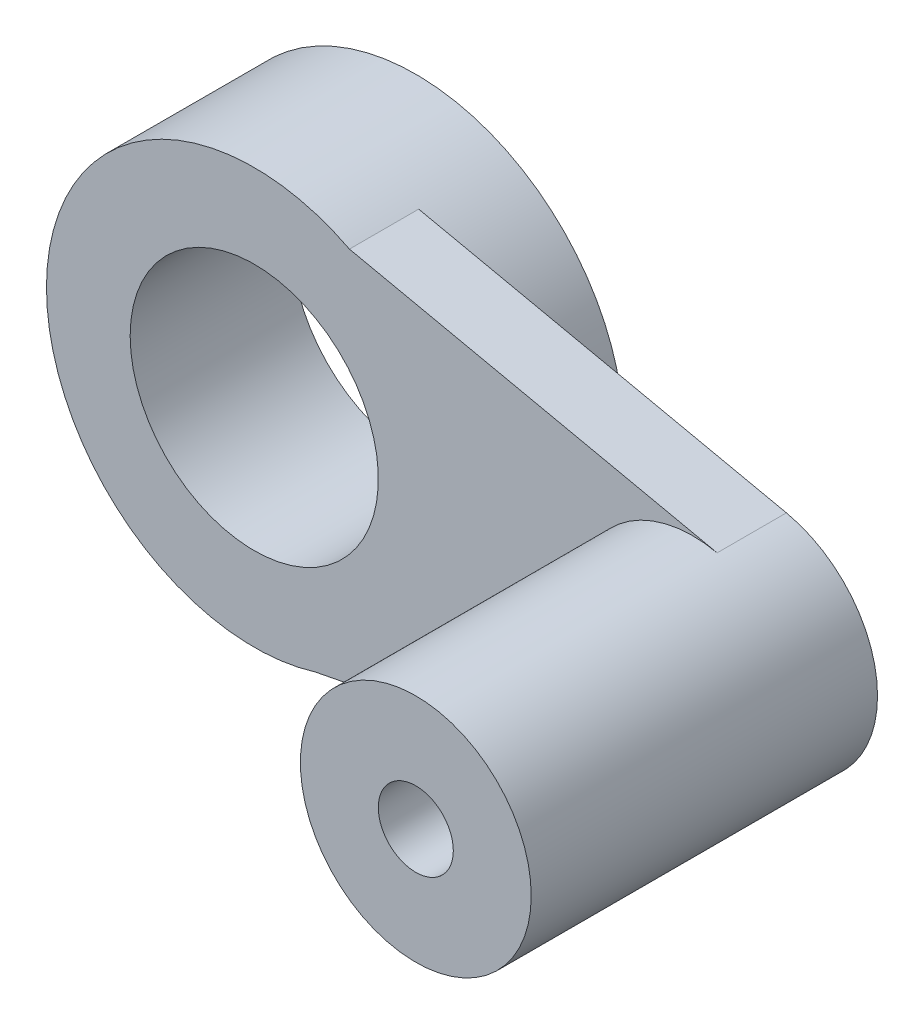
ISO-10303-21;
HEADER;
FILE_DESCRIPTION(('STEP AP214'),'2;1');
FILE_NAME('part.step','',(''),(''),'','','');
FILE_SCHEMA(('AUTOMOTIVE_DESIGN { 1 0 10303 214 1 1 1 1 }'));
ENDSEC;
DATA;
#1=APPLICATION_CONTEXT('core data for automotive mechanical design processes');
#2=APPLICATION_PROTOCOL_DEFINITION('international standard','automotive_design',2000,#1);
#3=PRODUCT_CONTEXT('',#1,'mechanical');
#4=PRODUCT('Part','Part','',(#3));
#5=PRODUCT_RELATED_PRODUCT_CATEGORY('part','',(#4));
#6=PRODUCT_DEFINITION_FORMATION('','',#4);
#7=PRODUCT_DEFINITION_CONTEXT('part definition',#1,'design');
#8=PRODUCT_DEFINITION('design','',#6,#7);
#9=PRODUCT_DEFINITION_SHAPE('','',#8);
#10=(LENGTH_UNIT() NAMED_UNIT(*) SI_UNIT(.MILLI.,.METRE.));
#11=(NAMED_UNIT(*) PLANE_ANGLE_UNIT() SI_UNIT($,.RADIAN.));
#12=(NAMED_UNIT(*) SI_UNIT($,.STERADIAN.) SOLID_ANGLE_UNIT());
#13=UNCERTAINTY_MEASURE_WITH_UNIT(LENGTH_MEASURE(1.E-05),#10,'distance_accuracy_value','');
#14=(GEOMETRIC_REPRESENTATION_CONTEXT(3) GLOBAL_UNCERTAINTY_ASSIGNED_CONTEXT((#13)) GLOBAL_UNIT_ASSIGNED_CONTEXT((#10,
#11,#12)) REPRESENTATION_CONTEXT('',''));
#15=CARTESIAN_POINT('',(0.,0.,0.));
#16=DIRECTION('',(0.,0.,1.));
#17=DIRECTION('',(1.,0.,0.));
#18=AXIS2_PLACEMENT_3D('',#15,#16,#17);
#19=CARTESIAN_POINT('',(0.,0.,-14000.));
#20=DIRECTION('',(0.,0.,1.));
#21=DIRECTION('',(1.,0.,0.));
#22=AXIS2_PLACEMENT_3D('',#19,#20,#21);
#23=CYLINDRICAL_SURFACE('',#22,18000.);
#24=DIRECTION('',(0.,0.,1.));
#25=VECTOR('',#24,1.);
#26=CARTESIAN_POINT('',(8246.21125123532,16000.,-6000.));
#27=LINE('',#26,#25);
#28=CARTESIAN_POINT('',(8246.21125123532,16000.,-6000.));
#29=VERTEX_POINT('',#28);
#30=CARTESIAN_POINT('',(8246.21125123532,16000.,0.));
#31=VERTEX_POINT('',#30);
#32=EDGE_CURVE('E97',#29,#31,#27,.T.);
#33=ORIENTED_EDGE('',*,*,#32,.F.);
#34=CARTESIAN_POINT('',(0.,0.,-6000.));
#35=DIRECTION('',(0.,0.,-1.));
#36=DIRECTION('',(1.,0.,0.));
#37=AXIS2_PLACEMENT_3D('',#34,#35,#36);
#38=CIRCLE('',#37,18000.);
#39=CARTESIAN_POINT('',(5281.40085752884,-17207.754210881,-6000.));
#40=VERTEX_POINT('',#39);
#41=EDGE_CURVE('E91',#29,#40,#38,.T.);
#42=ORIENTED_EDGE('',*,*,#41,.T.);
#43=DIRECTION('',(0.,0.,1.));
#44=VECTOR('',#43,1.);
#45=CARTESIAN_POINT('',(5281.40085752884,-17207.754210881,-6000.));
#46=LINE('',#45,#44);
#47=CARTESIAN_POINT('',(5281.40085752884,-17207.754210881,0.));
#48=VERTEX_POINT('',#47);
#49=EDGE_CURVE('E83',#40,#48,#46,.T.);
#50=ORIENTED_EDGE('',*,*,#49,.T.);
#51=CARTESIAN_POINT('',(0.,0.,0.));
#52=DIRECTION('',(0.,0.,1.));
#53=DIRECTION('',(1.,0.,0.));
#54=AXIS2_PLACEMENT_3D('',#51,#52,#53);
#55=CIRCLE('',#54,18000.);
#56=EDGE_CURVE('E42',#31,#48,#55,.T.);
#57=ORIENTED_EDGE('',*,*,#56,.F.);
#58=EDGE_LOOP('',(#33,#42,#50,#57));
#59=FACE_BOUND('',#58,.T.);
#60=CARTESIAN_POINT('',(0.,0.,-14000.));
#61=DIRECTION('',(0.,0.,1.));
#62=DIRECTION('',(1.,0.,0.));
#63=AXIS2_PLACEMENT_3D('',#60,#61,#62);
#64=CIRCLE('',#63,18000.);
#65=CARTESIAN_POINT('',(18000.,0.,-14000.));
#66=VERTEX_POINT('',#65);
#67=EDGE_CURVE('E11',#66,#66,#64,.T.);
#68=ORIENTED_EDGE('',*,*,#67,.T.);
#69=EDGE_LOOP('',(#68));
#70=FACE_BOUND('',#69,.T.);
#71=ADVANCED_FACE('F41',(#59,#70),#23,.T.);
#72=CARTESIAN_POINT('',(0.,0.,-14000.));
#73=DIRECTION('',(0.,0.,1.));
#74=DIRECTION('',(1.,0.,0.));
#75=AXIS2_PLACEMENT_3D('',#72,#73,#74);
#76=PLANE('',#75);
#77=CARTESIAN_POINT('',(0.,0.,-14000.));
#78=DIRECTION('',(0.,0.,-1.));
#79=DIRECTION('',(-1.,0.,0.));
#80=AXIS2_PLACEMENT_3D('',#77,#78,#79);
#81=CIRCLE('',#80,10750.);
#82=CARTESIAN_POINT('',(-10750.,0.,-14000.));
#83=VERTEX_POINT('',#82);
#84=EDGE_CURVE('E112',#83,#83,#81,.T.);
#85=ORIENTED_EDGE('',*,*,#84,.F.);
#86=EDGE_LOOP('',(#85));
#87=FACE_BOUND('',#86,.T.);
#88=ORIENTED_EDGE('',*,*,#67,.F.);
#89=EDGE_LOOP('',(#88));
#90=FACE_BOUND('',#89,.T.);
#91=ADVANCED_FACE('F125',(#87,#90),#76,.F.);
#92=CARTESIAN_POINT('',(0.,0.,0.));
#93=DIRECTION('',(0.,0.,1.));
#94=DIRECTION('',(1.,0.,0.));
#95=AXIS2_PLACEMENT_3D('',#92,#93,#94);
#96=PLANE('',#95);
#97=CARTESIAN_POINT('',(37994.6828068475,-635.67161887863,0.));
#98=DIRECTION('',(0.,0.,1.));
#99=DIRECTION('',(1.,0.,0.));
#100=AXIS2_PLACEMENT_3D('',#97,#98,#99);
#101=CIRCLE('',#100,10000.);
#102=CARTESIAN_POINT('',(40099.9459647422,9140.21028691437,0.));
#103=VERTEX_POINT('',#102);
#104=CARTESIAN_POINT('',(39720.1795834626,-10485.6797850626,0.));
#105=VERTEX_POINT('',#104);
#106=EDGE_CURVE('E102',#103,#105,#101,.T.);
#107=ORIENTED_EDGE('',*,*,#106,.F.);
#108=DIRECTION('',(-0.9775881905793,0.210526315789474,0.));
#109=VECTOR('',#108,1.);
#110=CARTESIAN_POINT('',(8246.21125123532,16000.,0.));
#111=LINE('',#110,#109);
#112=EDGE_CURVE('E99',#103,#31,#111,.T.);
#113=ORIENTED_EDGE('',*,*,#112,.T.);
#114=ORIENTED_EDGE('',*,*,#56,.T.);
#115=DIRECTION('',(0.981478201008145,0.191573852458563,0.));
#116=VECTOR('',#115,1.);
#117=CARTESIAN_POINT('',(5281.40085752884,-17207.754210881,0.));
#118=LINE('',#117,#116);
#119=EDGE_CURVE('E82',#48,#105,#118,.T.);
#120=ORIENTED_EDGE('',*,*,#119,.T.);
#121=EDGE_LOOP('',(#107,#113,#114,#120));
#122=FACE_BOUND('',#121,.T.);
#123=CARTESIAN_POINT('',(0.,0.,0.));
#124=DIRECTION('',(0.,0.,-1.));
#125=DIRECTION('',(-1.,0.,0.));
#126=AXIS2_PLACEMENT_3D('',#123,#124,#125);
#127=CIRCLE('',#126,10750.);
#128=CARTESIAN_POINT('',(-10750.,0.,0.));
#129=VERTEX_POINT('',#128);
#130=EDGE_CURVE('E111',#129,#129,#127,.T.);
#131=ORIENTED_EDGE('',*,*,#130,.T.);
#132=EDGE_LOOP('',(#131));
#133=FACE_BOUND('',#132,.T.);
#134=ADVANCED_FACE('F124',(#122,#133),#96,.T.);
#135=CARTESIAN_POINT('',(0.,0.,0.));
#136=DIRECTION('',(0.,0.,-1.));
#137=DIRECTION('',(-1.,0.,0.));
#138=AXIS2_PLACEMENT_3D('',#135,#136,#137);
#139=CYLINDRICAL_SURFACE('',#138,10750.);
#140=ORIENTED_EDGE('',*,*,#130,.F.);
#141=EDGE_LOOP('',(#140));
#142=FACE_BOUND('',#141,.T.);
#143=ORIENTED_EDGE('',*,*,#84,.T.);
#144=EDGE_LOOP('',(#143));
#145=FACE_BOUND('',#144,.T.);
#146=ADVANCED_FACE('F120',(#142,#145),#139,.F.);
#147=CARTESIAN_POINT('',(8246.21125123532,16000.,-6000.));
#148=DIRECTION('',(0.210526315789474,0.9775881905793,0.));
#149=DIRECTION('',(-0.977588190579301,0.210526315789474,0.));
#150=AXIS2_PLACEMENT_3D('',#147,#148,#149);
#151=PLANE('',#150);
#152=ORIENTED_EDGE('',*,*,#112,.F.);
#153=DIRECTION('',(0.,0.,1.));
#154=VECTOR('',#153,1.);
#155=CARTESIAN_POINT('',(40099.9459647422,9140.21028691437,-6000.));
#156=LINE('',#155,#154);
#157=CARTESIAN_POINT('',(40099.9459647422,9140.21028691437,-6000.));
#158=VERTEX_POINT('',#157);
#159=EDGE_CURVE('E90',#158,#103,#156,.T.);
#160=ORIENTED_EDGE('',*,*,#159,.F.);
#161=DIRECTION('',(-0.9775881905793,0.210526315789474,0.));
#162=VECTOR('',#161,1.);
#163=CARTESIAN_POINT('',(8246.21125123532,16000.,-6000.));
#164=LINE('',#163,#162);
#165=EDGE_CURVE('E89',#158,#29,#164,.T.);
#166=ORIENTED_EDGE('',*,*,#165,.T.);
#167=ORIENTED_EDGE('',*,*,#32,.T.);
#168=EDGE_LOOP('',(#152,#160,#166,#167));
#169=FACE_BOUND('',#168,.T.);
#170=ADVANCED_FACE('F150',(#169),#151,.T.);
#171=CARTESIAN_POINT('',(37994.6828068475,-635.67161887863,-6000.));
#172=DIRECTION('',(0.,0.,1.));
#173=DIRECTION('',(1.,0.,0.));
#174=AXIS2_PLACEMENT_3D('',#171,#172,#173);
#175=CYLINDRICAL_SURFACE('',#174,10000.);
#176=ORIENTED_EDGE('',*,*,#159,.T.);
#177=ORIENTED_EDGE('',*,*,#106,.T.);
#178=DIRECTION('',(0.,0.,1.));
#179=VECTOR('',#178,1.);
#180=CARTESIAN_POINT('',(39720.1795834626,-10485.6797850626,-6000.));
#181=LINE('',#180,#179);
#182=CARTESIAN_POINT('',(39720.1795834626,-10485.6797850626,-6000.));
#183=VERTEX_POINT('',#182);
#184=EDGE_CURVE('E54',#105,#183,#181,.F.);
#185=ORIENTED_EDGE('',*,*,#184,.T.);
#186=CARTESIAN_POINT('',(37994.6828068475,-635.67161887863,-6000.));
#187=DIRECTION('',(0.,0.,1.));
#188=DIRECTION('',(1.,0.,0.));
#189=AXIS2_PLACEMENT_3D('',#186,#187,#188);
#190=CIRCLE('',#189,10000.);
#191=EDGE_CURVE('E64',#183,#158,#190,.T.);
#192=ORIENTED_EDGE('',*,*,#191,.T.);
#193=EDGE_LOOP('',(#176,#177,#185,#192));
#194=FACE_BOUND('',#193,.T.);
#195=CARTESIAN_POINT('',(37994.6828068475,-635.67161887863,24000.));
#196=DIRECTION('',(0.,0.,1.));
#197=DIRECTION('',(1.,0.,0.));
#198=AXIS2_PLACEMENT_3D('',#195,#196,#197);
#199=CIRCLE('',#198,10000.);
#200=CARTESIAN_POINT('',(47994.6828068475,-635.67161887863,24000.));
#201=VERTEX_POINT('',#200);
#202=EDGE_CURVE('E231',#201,#201,#199,.T.);
#203=ORIENTED_EDGE('',*,*,#202,.F.);
#204=EDGE_LOOP('',(#203));
#205=FACE_BOUND('',#204,.T.);
#206=ADVANCED_FACE('F147',(#194,#205),#175,.T.);
#207=CARTESIAN_POINT('',(5281.40085752884,-17207.754210881,-6000.));
#208=DIRECTION('',(0.191573852458563,-0.981478201008145,0.));
#209=DIRECTION('',(0.981478201008145,0.191573852458563,0.));
#210=AXIS2_PLACEMENT_3D('',#207,#208,#209);
#211=PLANE('',#210);
#212=ORIENTED_EDGE('',*,*,#184,.F.);
#213=ORIENTED_EDGE('',*,*,#119,.F.);
#214=ORIENTED_EDGE('',*,*,#49,.F.);
#215=DIRECTION('',(0.981478201008145,0.191573852458563,0.));
#216=VECTOR('',#215,1.);
#217=CARTESIAN_POINT('',(5281.40085752884,-17207.754210881,-6000.));
#218=LINE('',#217,#216);
#219=EDGE_CURVE('E81',#40,#183,#218,.T.);
#220=ORIENTED_EDGE('',*,*,#219,.T.);
#221=EDGE_LOOP('',(#212,#213,#214,#220));
#222=FACE_BOUND('',#221,.T.);
#223=ADVANCED_FACE('F85',(#222),#211,.T.);
#224=CARTESIAN_POINT('',(0.,0.,-6000.));
#225=DIRECTION('',(0.,0.,1.));
#226=DIRECTION('',(1.,0.,0.));
#227=AXIS2_PLACEMENT_3D('',#224,#225,#226);
#228=PLANE('',#227);
#229=CARTESIAN_POINT('',(37994.6828068475,-635.67161887863,-6000.));
#230=DIRECTION('',(0.,0.,1.));
#231=DIRECTION('',(1.,0.,0.));
#232=AXIS2_PLACEMENT_3D('',#229,#230,#231);
#233=CIRCLE('',#232,3250.);
#234=CARTESIAN_POINT('',(41244.6828068475,-635.67161887863,-6000.));
#235=VERTEX_POINT('',#234);
#236=EDGE_CURVE('E235',#235,#235,#233,.T.);
#237=ORIENTED_EDGE('',*,*,#236,.T.);
#238=EDGE_LOOP('',(#237));
#239=FACE_BOUND('',#238,.T.);
#240=ORIENTED_EDGE('',*,*,#165,.F.);
#241=ORIENTED_EDGE('',*,*,#191,.F.);
#242=ORIENTED_EDGE('',*,*,#219,.F.);
#243=ORIENTED_EDGE('',*,*,#41,.F.);
#244=EDGE_LOOP('',(#240,#241,#242,#243));
#245=FACE_BOUND('',#244,.T.);
#246=ADVANCED_FACE('F95',(#239,#245),#228,.F.);
#247=CARTESIAN_POINT('',(37994.6828068475,-635.67161887863,24000.));
#248=DIRECTION('',(0.,0.,1.));
#249=DIRECTION('',(1.,0.,0.));
#250=AXIS2_PLACEMENT_3D('',#247,#248,#249);
#251=PLANE('',#250);
#252=CARTESIAN_POINT('',(37994.6828068475,-635.67161887863,24000.));
#253=DIRECTION('',(0.,0.,1.));
#254=DIRECTION('',(1.,0.,0.));
#255=AXIS2_PLACEMENT_3D('',#252,#253,#254);
#256=CIRCLE('',#255,3250.);
#257=CARTESIAN_POINT('',(41244.6828068475,-635.67161887863,24000.));
#258=VERTEX_POINT('',#257);
#259=EDGE_CURVE('E228',#258,#258,#256,.T.);
#260=ORIENTED_EDGE('',*,*,#259,.F.);
#261=EDGE_LOOP('',(#260));
#262=FACE_BOUND('',#261,.T.);
#263=ORIENTED_EDGE('',*,*,#202,.T.);
#264=EDGE_LOOP('',(#263));
#265=FACE_BOUND('',#264,.T.);
#266=ADVANCED_FACE('F175',(#262,#265),#251,.T.);
#267=CARTESIAN_POINT('',(37994.6828068475,-635.67161887863,-14000.));
#268=DIRECTION('',(0.,0.,1.));
#269=DIRECTION('',(1.,0.,0.));
#270=AXIS2_PLACEMENT_3D('',#267,#268,#269);
#271=CYLINDRICAL_SURFACE('',#270,3250.);
#272=ORIENTED_EDGE('',*,*,#259,.T.);
#273=EDGE_LOOP('',(#272));
#274=FACE_BOUND('',#273,.T.);
#275=ORIENTED_EDGE('',*,*,#236,.F.);
#276=EDGE_LOOP('',(#275));
#277=FACE_BOUND('',#276,.T.);
#278=ADVANCED_FACE('F181',(#274,#277),#271,.F.);
#279=CLOSED_SHELL('',(#71,#91,#134,#146,#170,#206,#223,#246,#266,#278));
#280=MANIFOLD_SOLID_BREP('B2',#279);
#281=ADVANCED_BREP_SHAPE_REPRESENTATION('',(#18,#280),#14);
#282=SHAPE_DEFINITION_REPRESENTATION(#9,#281);
ENDSEC;
END-ISO-10303-21;
